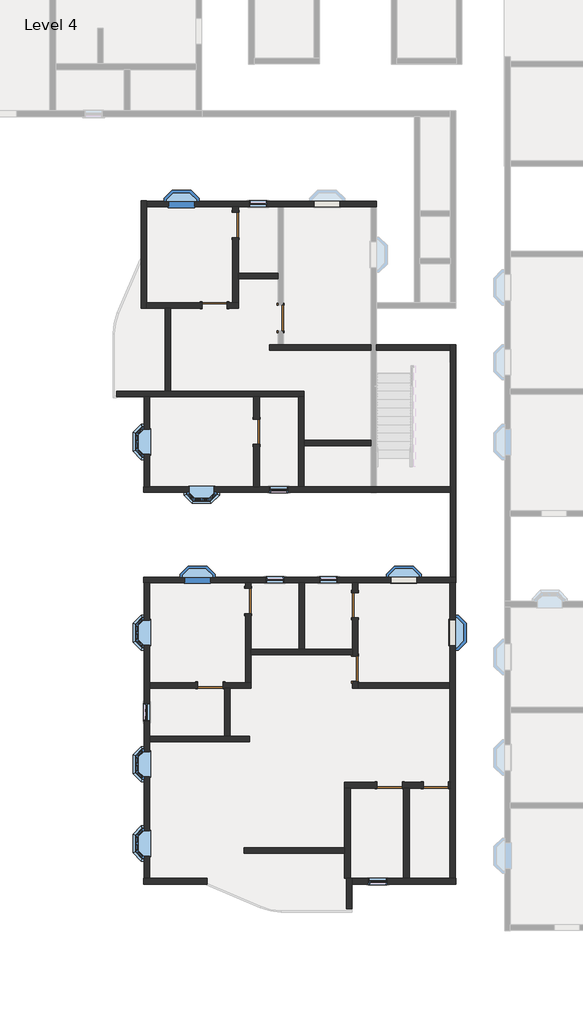
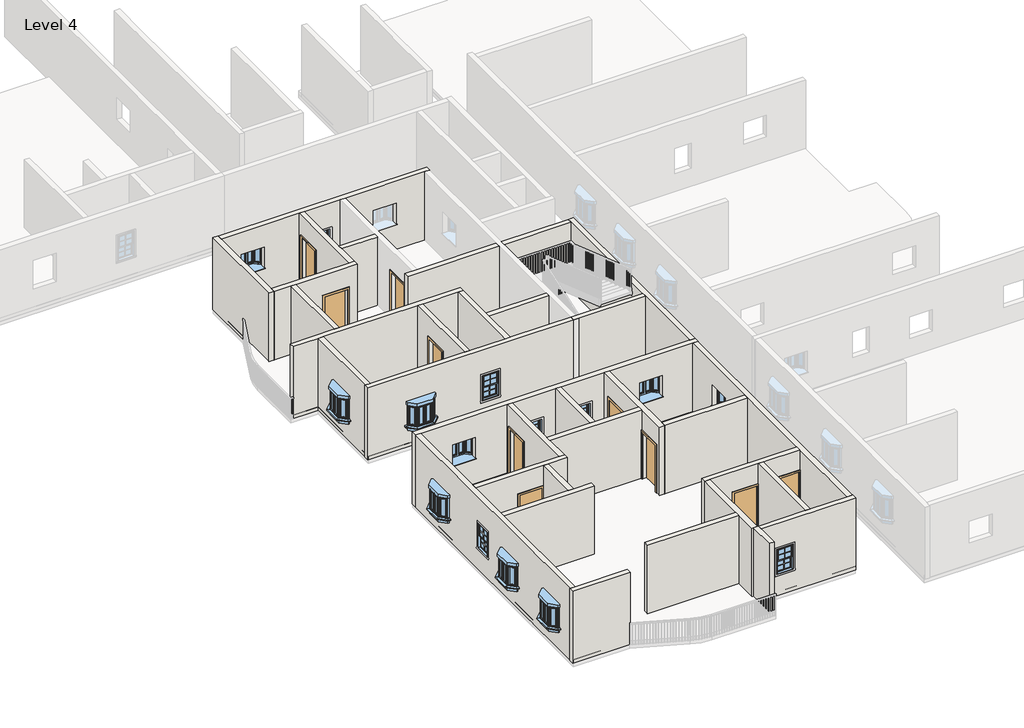
# One storey, part 1 of 14: 32 walls, 15 windows, 10 doors.
# Revit data of these elements (continued)
# Element 54 (IfcWindow, "Window-Double-Hung : 26\" x 42\"") (continued)
#   Window Inset = 0' - 0"
#   Interior Wall Closure = 0' - 1 1/2"
#   Frame Extension = 0' - 1 1/4"
#   Exterior Wall Closure = 0' - 0 1/2"
#   Interior Trim Visibility = yes
#   Indicator Visibility = yes
#   Exterior Trim Visibility = yes
#   Phase Created = New Construction
#   Materials on its faces: "Wood - Stained", "Glass", "Clad - White"
# Element 55 (IfcWindow, "Window-Double-Hung : 26\" x 42\"")
#   Mark = "215"
#   Window Inset = 0' - 0"
#   Interior Wall Closure = 0' - 1 1/2"
#   Frame Extension = 0' - 1 1/4"
#   Exterior Wall Closure = 0' - 0 1/2"
#   Interior Trim Visibility = yes
#   Indicator Visibility = yes
#   Exterior Trim Visibility = yes
#   Phase Created = New Construction
#   Materials on its faces: "Wood - Stained", "Glass", "Clad - White"
# Element 56 (IfcWindow, "Window-Double-Hung : 26\" x 42\"")
#   Mark = "216"
#   Window Inset = 0' - 0"
#   Interior Wall Closure = 0' - 1 1/2"
#   Frame Extension = 0' - 1 1/4"
#   Exterior Wall Closure = 0' - 0 1/2"
#   Interior Trim Visibility = yes
#   Indicator Visibility = yes
#   Exterior Trim Visibility = yes
#   Phase Created = New Construction
#   Materials on its faces: "Wood - Stained", "Glass", "Clad - White"
# Element 57 (IfcWindow, "Window-Double-Hung : 26\" x 42\"")
#   Mark = "217"
#   Window Inset = 0' - 0"
#   Interior Wall Closure = 0' - 1 1/2"
#   Frame Extension = 0' - 1 1/4"
#   Exterior Wall Closure = 0' - 0 1/2"
#   Interior Trim Visibility = yes
#   Indicator Visibility = yes
#   Exterior Trim Visibility = yes
#   Phase Created = New Construction
#   Materials on its faces: "Wood - Stained", "Glass", "Clad - White"
# Materials
#   "Door - Panel": class "Wood", colour RGB 210 159 95, transparency 0, Cost = 0
#   "Door - Frame": colour RGB 118 70 51, transparency 0, Cost = 0
#   "Window Frame": colour RGB 249 249 249, transparency 0
#   "Glass": class "Glass", colour RGB 0 128 192, transparency 0.75, Description = "Soda Lime Glass", Cost = 0
#   "Wood - Stained": class "Wood", colour RGB 224 178 126, transparency 0, Cost = 0
#   "Clad - White": class "Wood", colour RGB 242 242 238, transparency 0, Cost = 0
#   "Default Wall": colour RGB 128 128 128, transparency 0, Cost = 0
#   "Earth": class "Generic", colour RGB 97 75 62, transparency 0, Description = "Soil", Cost = 0
#   "Parking Stripe": class "Paint", colour RGB 250 250 91, transparency 0, Cost = 0
#   "Carpet (1)": class "Carpet", colour RGB 124 80 67, transparency 0, Description = "Interior finish", Cost = 0
#   "Softwood, Lumber": class "Wood", colour RGB 223 192 134, transparency 0, Description = "Pinus Echinata", Cost = 0
